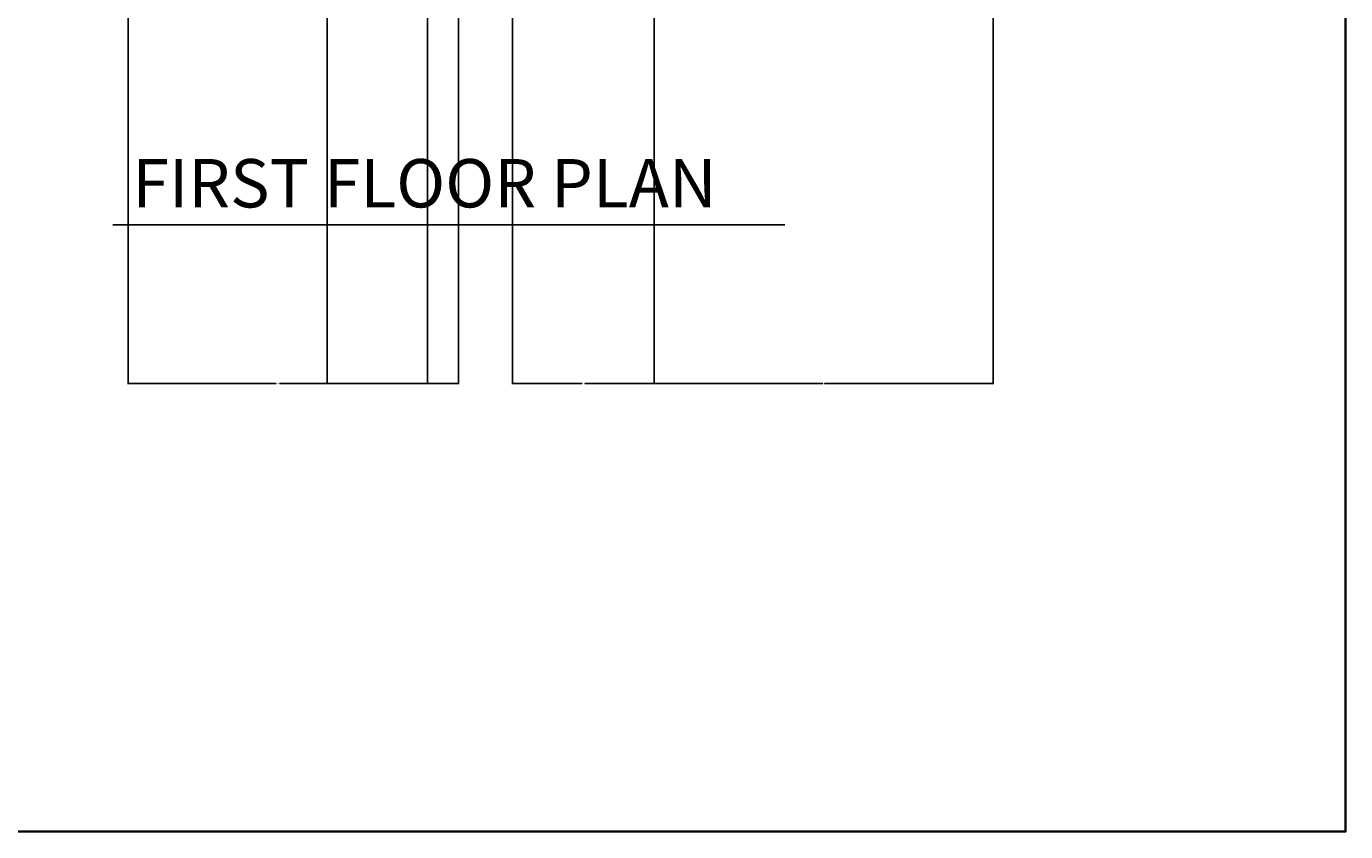
# Model space of a CAD drawing. Units: inches. Extents: x 1734 to 2405, y 1500 to 2491.
# Tile 8 of 14: x 2078 to 2405, y 1500 to 1700. Entities that reach past the tile are written whole.
import ezdxf

# ---------------------------------------------------------------- set-up
doc = ezdxf.new("R2010")
doc.units = ezdxf.units.IN
for name, color, linetype, lineweight in [('A-ANNO-DIMS', 2, 'Continuous', 18), ('A-ANNO-TITL', 7, 'Continuous', 25), ('A-ANNO-TTLB', 7, 'Continuous', 35)]:
    doc.layers.add(name, color=color, linetype=linetype, lineweight=lineweight)
doc.styles.get("Standard").update_dxf_attribs({"font": 'arial.ttf'})
doc.dimstyles.get("Standard").update_dxf_attribs({"dimtxt": 0.18, "dimasz": 0.18, "dimexe": 0.18, "dimexo": 0.0625, "dimgap": 0.09, "dimtad": 0, "dimtih": 1, "dimtoh": 1, "dimdec": 4, "dimzin": 0, "dimdsep": 46, "dimtxsty": 'Standard', "dimcen": 0.09, "dimadec": 0, "dimazin": 0, "dimtfac": 1, "dimtdec": 4, "dimtofl": 0, "dimtmove": 0, "dimatfit": 3, "dimfxl": 1, "dimtolj": 1, "dimtzin": 0, "dimarcsym": 0})

# ---------------------------------------------------------------- blocks, each defined once
blk = doc.blocks.new('*D41')
at = {"layer": 'A-ANNO-DIMS', "color": 0, "lineweight": -2, "transparency": 16777216}
for p, q in [((2233.24, 1956.26), (2233.24, 1611.24)), ((2317.24, 1956.26), (2317.24, 1611.24)), ((2233.42, 1611.42), (2275.03, 1611.42)), ((2317.06, 1611.42), (2275.46, 1611.42))]:
    blk.add_line(p, q, dxfattribs=at)
at = {"layer": 'A-ANNO-DIMS', "color": 0, "transparency": 16777216}
for points in [[(2233.42, 1611.45), (2233.42, 1611.39), (2233.24, 1611.42)], [(2317.06, 1611.45), (2317.06, 1611.39), (2317.24, 1611.42)]]:
    blk.add_solid(points, dxfattribs=at)
at = {"layer": 'Defpoints', "color": 0, "transparency": 16777216}
for p in [(2233.24, 1956.32), (2317.24, 1956.32), (2317.24, 1611.42)]:
    blk.add_point(p, dxfattribs=at)
at = {"layer": 'A-ANNO-DIMS', "color": 0, "transparency": 16777216, "insert": (2275.24, 1611.42), "char_height": 0.18, "attachment_point": 5}
blk.add_mtext('\\A1;84', dxfattribs=at)
blk = doc.blocks.new('*D42')
at = {"layer": 'A-ANNO-DIMS', "color": 0, "lineweight": -2, "transparency": 16777216}
for p, q in [((2152.2, 2198.26), (2152.2, 1611.24)), ((2184.72, 2198.26), (2184.72, 1611.24)), ((2152.38, 1611.42), (2168, 1611.42)), ((2184.54, 1611.42), (2168.92, 1611.42))]:
    blk.add_line(p, q, dxfattribs=at)
at = {"layer": 'A-ANNO-DIMS', "color": 0, "transparency": 16777216}
for points in [[(2152.38, 1611.45), (2152.38, 1611.39), (2152.2, 1611.42)], [(2184.54, 1611.45), (2184.54, 1611.39), (2184.72, 1611.42)]]:
    blk.add_solid(points, dxfattribs=at)
at = {"layer": 'Defpoints', "color": 0, "transparency": 16777216}
for p in [(2152.2, 2198.32), (2184.72, 2198.32), (2184.72, 1611.42)]:
    blk.add_point(p, dxfattribs=at)
at = {"layer": 'A-ANNO-DIMS', "color": 0, "transparency": 16777216, "insert": (2168.46, 1611.42), "char_height": 0.18, "attachment_point": 5}
blk.add_mtext('\\A1;32.526', dxfattribs=at)
blk = doc.blocks.new('*D43')
at = {"layer": 'A-ANNO-DIMS', "color": 0, "lineweight": -2, "transparency": 16777216}
for p, q in [((2233.24, 2200.45), (2233.24, 1611.24)), ((2198.08, 2198.26), (2198.08, 1611.24)), ((2198.26, 1611.42), (2215.27, 1611.42)), ((2233.06, 1611.42), (2216.05, 1611.42))]:
    blk.add_line(p, q, dxfattribs=at)
at = {"layer": 'A-ANNO-DIMS', "color": 0, "transparency": 16777216}
for points in [[(2198.26, 1611.45), (2198.26, 1611.39), (2198.08, 1611.42)], [(2233.06, 1611.45), (2233.06, 1611.39), (2233.24, 1611.42)]]:
    blk.add_solid(points, dxfattribs=at)
at = {"layer": 'Defpoints', "color": 0, "transparency": 16777216}
for p in [(2233.24, 2200.51), (2198.08, 2198.32), (2233.24, 1611.42)]:
    blk.add_point(p, dxfattribs=at)
at = {"layer": 'A-ANNO-DIMS', "color": 0, "transparency": 16777216, "insert": (2215.66, 1611.42), "char_height": 0.18, "attachment_point": 5}
blk.add_mtext('\\A1;35.17', dxfattribs=at)
blk = doc.blocks.new('*D44')
at = {"layer": 'A-ANNO-DIMS', "color": 0, "lineweight": -2, "transparency": 16777216}
for p, q in [((2102.87, 2356.76), (2102.87, 1611.24)), ((2177.04, 2356.76), (2177.04, 1611.24)), ((2103.05, 1611.42), (2139.56, 1611.42)), ((2176.86, 1611.42), (2140.35, 1611.42))]:
    blk.add_line(p, q, dxfattribs=at)
at = {"layer": 'A-ANNO-DIMS', "color": 0, "transparency": 16777216}
for points in [[(2103.05, 1611.45), (2103.05, 1611.39), (2102.87, 1611.42)], [(2176.86, 1611.45), (2176.86, 1611.39), (2177.04, 1611.42)]]:
    blk.add_solid(points, dxfattribs=at)
at = {"layer": 'Defpoints', "color": 0, "transparency": 16777216}
for p in [(2102.87, 2356.82), (2177.04, 2356.82), (2177.04, 1611.42)]:
    blk.add_point(p, dxfattribs=at)
at = {"layer": 'A-ANNO-DIMS', "color": 0, "transparency": 16777216, "insert": (2139.96, 1611.42), "char_height": 0.18, "attachment_point": 5}
blk.add_mtext('\\A1;74.17', dxfattribs=at)

msp = doc.modelspace()

# ---------------------------------------------------------------- linework, layer by layer
at = {"layer": 'A-ANNO-TITL'}
msp.add_line((2265.5698, 1650.7736), (2099.0443, 1650.7736), dxfattribs=at)
at = {"layer": 'A-ANNO-TTLB'}
msp.add_lwpolyline([(1734.1307, 2491.1293), (2404.5589, 2491.1293), (2404.5589, 1500.293), (1734.1307, 1500.293)], close=True, dxfattribs=at)

# ---------------------------------------------------------------- texts
at = {"layer": 'A-ANNO-TITL', "insert": (2103.9125, 1667.0663), "char_height": 12, "attachment_point": 1}
msp.add_mtext_dynamic_manual_height_columns('FIRST FLOOR PLAN', width=206.72645, gutter_width=12.5, heights=[0], dxfattribs=at)

# ---------------------------------------------------------------- dimensions: what is measured, and where the dimension line sits
at = {"layer": 'A-ANNO-DIMS'}
for base, p1, p2, override, picture, middle in [((2177.0411, 1611.4236), (2102.8692, 2356.8246), (2177.0411, 2356.8246), {"dimdec": 2, "dimlfac": 1, "dimrnd": 0, "dimzin": 0, "dimdsep": 46, "dimlunit": 2}, '*D44', (2139.9551, 1611.4236)), ((2233.2445, 1611.4236), (2198.0776, 2198.3246), (2233.2445, 2200.5102), {"dimdec": 2, "dimlfac": 1, "dimrnd": 0, "dimzin": 0, "dimdsep": 46, "dimlunit": 2}, '*D43', (2215.661, 1611.4236)), ((2184.7241, 1611.4236), (2152.1978, 2198.3246), (2184.7241, 2198.3246), {"dimdec": 3, "dimlfac": 1, "dimrnd": 0, "dimzin": 0, "dimdsep": 46, "dimlunit": 2}, '*D42', (2168.461, 1611.4236)), ((2317.2445, 1611.4236), (2233.2445, 1956.3246), (2317.2445, 1956.3246), {"dimdec": 0, "dimlfac": 1, "dimrnd": 0, "dimzin": 0, "dimdsep": 46, "dimlunit": 2}, '*D41', (2275.2445, 1611.4236))]:
    dim = msp.add_linear_dim(base=base, p1=p1, p2=p2, dimstyle='Standard', override=override, dxfattribs=at)
    dim.commit()
    dim.dimension.update_dxf_attribs({"geometry": picture, "text_midpoint": middle})

doc.saveas('drawing.dxf')
